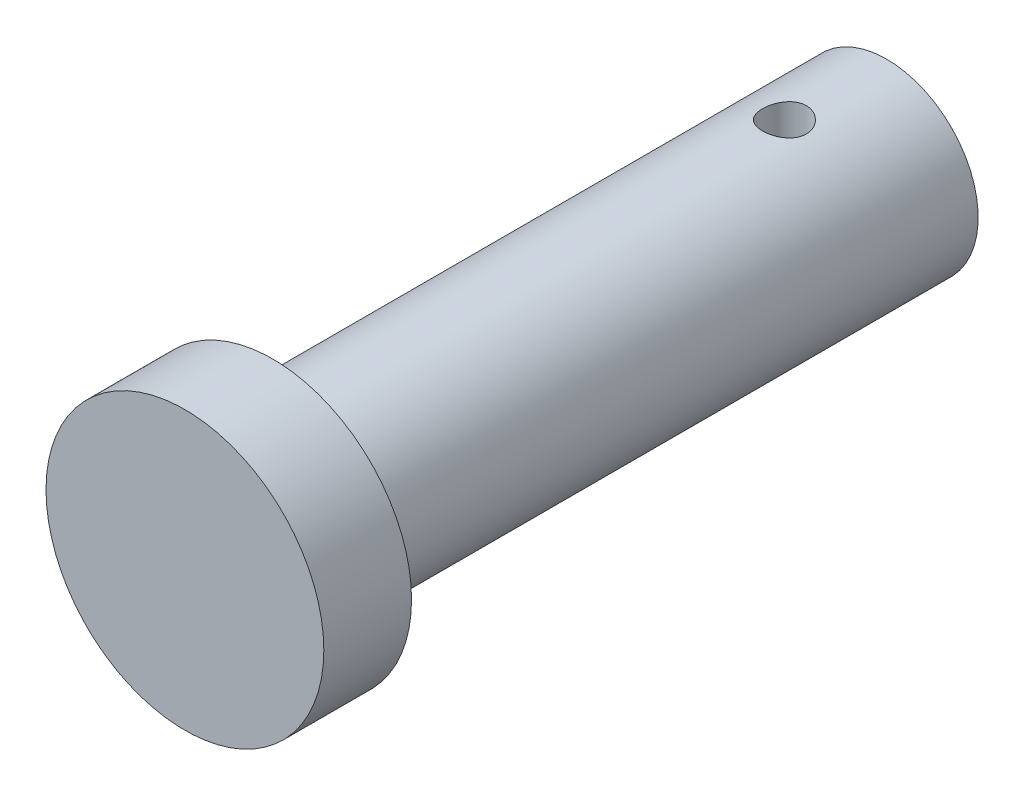
from build123d import *

# Parameters (mm, degrees)
HEAD_PROFILE_38_R      = 19
HEAD_38X12_DEPTH       = 12
SHANK_PROFILE_25_R     = 12.5
SHANK_25X84_DEPTH      = 84
CROSS_HOLE_PROFILE_6_R = 3
CROSS_HOLE_6_DEPTH     = 42


with BuildPart() as part:
    # Head Profile Ø38 → Head Ø38x12 (new body)
    with BuildSketch(Plane.XY):
        Circle(HEAD_PROFILE_38_R)
    extrude(amount=HEAD_38X12_DEPTH)

    # Shank Profile Ø25 → Shank Ø25x84 (add)
    with BuildSketch(Plane(origin=(0, 0, 0), x_dir=(-1, 0, 0), z_dir=(0, 0, -1))):
        with Locations(Location((0, 0, 0), (0, 0, 180))):
            Circle(SHANK_PROFILE_25_R)
    extrude(amount=SHANK_25X84_DEPTH)

    # Cross Hole Profile Ø6 → Cross Hole Ø6 (cut, symmetric)
    with BuildSketch(Plane(origin=(0, 0, 0), x_dir=(1, 0, 0), z_dir=(0, 1, 0))):
        with Locations(Location((0, 70, 0), (0, 0, 270))):
            Circle(CROSS_HOLE_PROFILE_6_R)
    extrude(amount=CROSS_HOLE_6_DEPTH, both=True, mode=Mode.SUBTRACT)


solid = part.part
